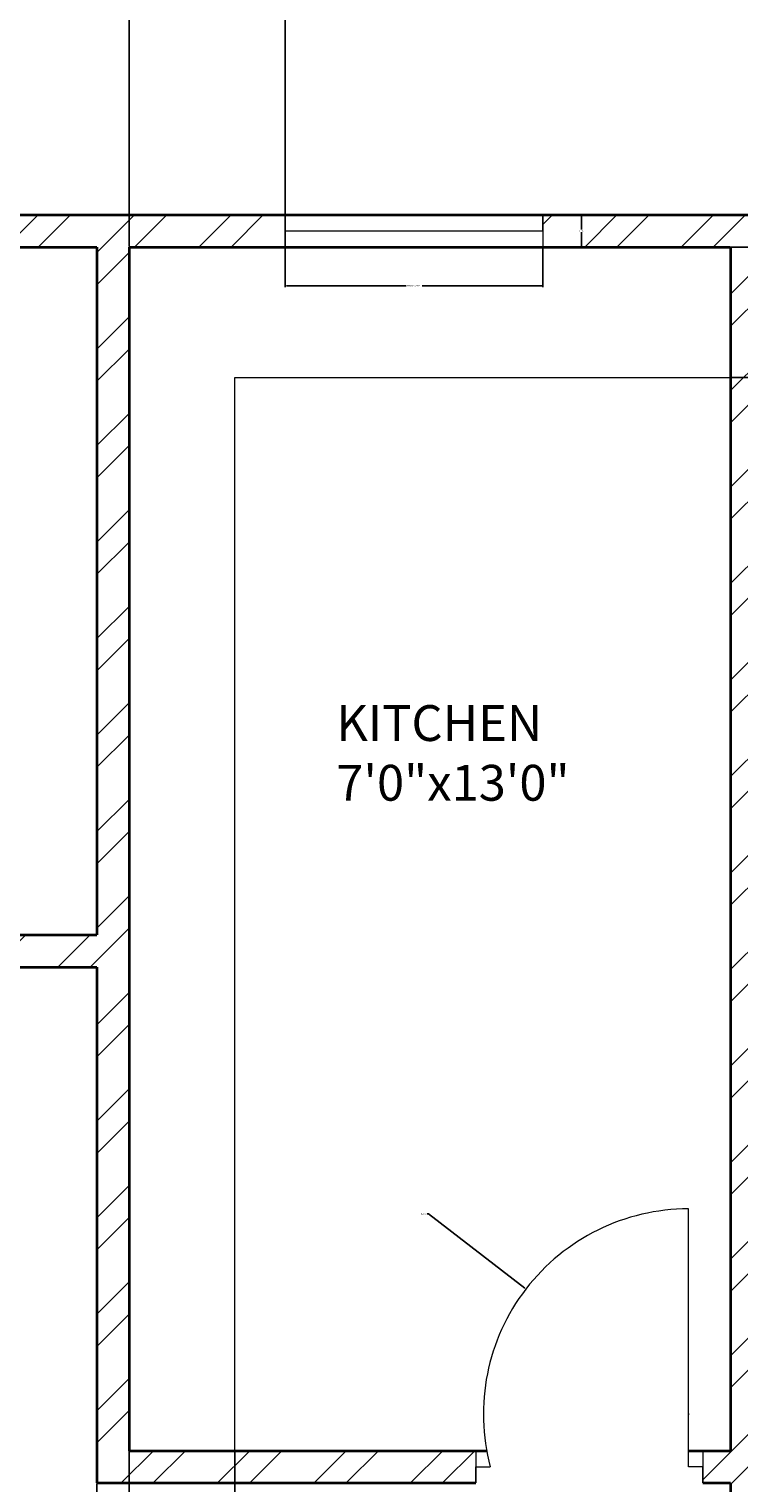
# Model space of a CAD drawing. Units: inches. Extents: x 392 to 1254, y 1207 to 2665.
# Tile 10 of 15: x 733 to 832, y 2052 to 2255. Entities that reach past the tile are written whole.
import ezdxf

# ---------------------------------------------------------------- set-up
doc = ezdxf.new("R2010")
doc.units = ezdxf.units.IN
for name, color, linetype, lineweight in [('A-ANNO-DIMS', 2, 'Continuous', 18), ('A-AREA-IDEN', 7, 'Continuous', 18), ('A-DOOR', 3, 'Continuous', 18), ('A-FLOR-FIXT', 9, 'Continuous', 18), ('A-GLAZ', 4, 'Continuous', 18), ('A-WALL', 7, 'Continuous', 35), ('A-WALL-PATT', 252, 'Continuous', 13)]:
    doc.layers.add(name, color=color, linetype=linetype, lineweight=lineweight)
doc.styles.get("Standard").update_dxf_attribs({"font": 'arial.ttf'})
doc.dimstyles.get("Standard").update_dxf_attribs({"dimtxt": 0.18, "dimasz": 0.18, "dimexe": 0.18, "dimexo": 0.0625, "dimgap": 0.09, "dimtad": 0, "dimtih": 1, "dimtoh": 1, "dimdec": 4, "dimzin": 0, "dimdsep": 46, "dimtxsty": 'Standard', "dimcen": 0.09, "dimadec": 0, "dimazin": 0, "dimtfac": 1, "dimtdec": 4, "dimtofl": 0, "dimtmove": 0, "dimatfit": 3, "dimfxl": 1, "dimtolj": 1, "dimtzin": 0, "dimarcsym": 0})

# ---------------------------------------------------------------- blocks, each defined once
blk = doc.blocks.new('WIN-36')
for p, q in [((0, 0), (0, 4.5)), ((0, 4.5), (0, 2.25)), ((36, 2.25), (36, 4.5)), ((36, 4.5), (36, 0)), ((0, 2.25), (36, 2.25))]:
    blk.add_line(p, q)
blk = doc.blocks.new('*D23')
at = {"layer": 'A-ANNO-DIMS', "color": 0, "lineweight": -2, "transparency": 16777216}
for p, q in [((768.58, 2224.73), (768.58, 2219.22)), ((804.58, 2224.73), (804.58, 2219.22)), ((768.76, 2219.4), (785.46, 2219.4)), ((804.4, 2219.4), (787.7, 2219.4))]:
    blk.add_line(p, q, dxfattribs=at)
at = {"layer": 'A-ANNO-DIMS', "color": 0, "transparency": 16777216}
for points in [[(768.76, 2219.43), (768.76, 2219.37), (768.58, 2219.4)], [(804.4, 2219.43), (804.4, 2219.37), (804.58, 2219.4)]]:
    blk.add_solid(points, dxfattribs=at)
at = {"layer": 'Defpoints', "color": 0, "transparency": 16777216}
for p in [(768.58, 2224.8), (804.58, 2224.8), (804.58, 2219.4)]:
    blk.add_point(p, dxfattribs=at)
at = {"layer": 'A-ANNO-DIMS', "color": 0, "transparency": 16777216, "insert": (786.58, 2219.4), "char_height": 0.18, "attachment_point": 5}
blk.add_mtext('\\A1;WINDOW 36 TYP.', dxfattribs=at)
blk = doc.blocks.new('*D24')
at = {"layer": 'A-ANNO-DIMS', "color": 0, "lineweight": -2, "transparency": 16777216}
for p, q in [((804.64, 2229.3), (810.16, 2229.3)), ((809.98, 2229.12), (809.98, 2227.23)), ((809.98, 2224.98), (809.98, 2226.86)), ((804.64, 2224.8), (810.16, 2224.8))]:
    blk.add_line(p, q, dxfattribs=at)
at = {"layer": 'A-ANNO-DIMS', "color": 0, "transparency": 16777216}
for points in [[(809.95, 2229.12), (810.01, 2229.12), (809.98, 2229.3)], [(809.95, 2224.98), (810.01, 2224.98), (809.98, 2224.8)]]:
    blk.add_solid(points, dxfattribs=at)
at = {"layer": 'Defpoints', "color": 0, "transparency": 16777216}
for p in [(804.58, 2229.3), (809.98, 2229.3), (804.58, 2224.8)]:
    blk.add_point(p, dxfattribs=at)
at = {"layer": 'A-ANNO-DIMS', "color": 0, "transparency": 16777216, "insert": (809.98, 2227.05), "char_height": 0.18, "attachment_point": 5}
blk.add_mtext('\\A1;5 TYP.', dxfattribs=at)
blk = doc.blocks.new('*D26')
at = {"layer": 'A-ANNO-DIMS', "color": 0, "lineweight": -2, "transparency": 16777216}
for p, q in [((541.22, 2229.3), (495, 2229.3)), ((495.18, 2229.12), (495.18, 1819.98)), ((495.18, 1410.48), (495.18, 1819.61)), ((753.23, 1410.3), (495, 1410.3))]:
    blk.add_line(p, q, dxfattribs=at)
at = {"layer": 'A-ANNO-DIMS', "color": 0, "transparency": 16777216}
for points in [[(495.15, 2229.12), (495.21, 2229.12), (495.18, 2229.3)], [(495.15, 1410.48), (495.21, 1410.48), (495.18, 1410.3)]]:
    blk.add_solid(points, dxfattribs=at)
at = {"layer": 'Defpoints', "color": 0, "transparency": 16777216}
for p in [(495.18, 2229.3), (541.28, 2229.3), (753.29, 1410.3)]:
    blk.add_point(p, dxfattribs=at)
at = {"layer": 'A-ANNO-DIMS', "color": 0, "transparency": 16777216, "insert": (495.18, 1819.8), "char_height": 0.18, "attachment_point": 5}
blk.add_mtext('\\A1;819', dxfattribs=at)
blk = doc.blocks.new('*D75')
at = {"layer": 'A-ANNO-DIMS', "color": 0, "lineweight": -2, "transparency": 16777216}
for p, q in [((746.78, 2056.73), (746.78, 1364.02)), ((742.28, 2052.23), (742.28, 1364.02)), ((742.46, 1364.2), (744.27, 1364.2)), ((746.6, 1364.2), (744.79, 1364.2))]:
    blk.add_line(p, q, dxfattribs=at)
at = {"layer": 'A-ANNO-DIMS', "color": 0, "transparency": 16777216}
for points in [[(742.46, 1364.23), (742.46, 1364.17), (742.28, 1364.2)], [(746.6, 1364.23), (746.6, 1364.17), (746.78, 1364.2)]]:
    blk.add_solid(points, dxfattribs=at)
at = {"layer": 'Defpoints', "color": 0, "transparency": 16777216}
for p in [(746.78, 2056.8), (742.28, 2052.3), (746.78, 1364.2)]:
    blk.add_point(p, dxfattribs=at)
at = {"layer": 'A-ANNO-DIMS', "color": 0, "transparency": 16777216, "insert": (744.53, 1364.2), "char_height": 0.18, "attachment_point": 5}
blk.add_mtext('\\A1;4.5', dxfattribs=at)
blk = doc.blocks.new('*D77')
at = {"layer": 'A-ANNO-DIMS', "color": 0, "lineweight": -2, "transparency": 16777216}
for p, q in [((746.78, 2224.86), (746.78, 2297.33)), ((768.58, 2224.86), (768.58, 2297.33)), ((746.96, 2297.15), (757.21, 2297.15)), ((768.4, 2297.15), (758.14, 2297.15))]:
    blk.add_line(p, q, dxfattribs=at)
at = {"layer": 'A-ANNO-DIMS', "color": 0, "transparency": 16777216}
for points in [[(746.96, 2297.18), (746.96, 2297.12), (746.78, 2297.15)], [(768.4, 2297.18), (768.4, 2297.12), (768.58, 2297.15)]]:
    blk.add_solid(points, dxfattribs=at)
at = {"layer": 'Defpoints', "color": 0, "transparency": 16777216}
for p in [(768.58, 2297.15), (746.78, 2224.8), (768.58, 2224.8)]:
    blk.add_point(p, dxfattribs=at)
at = {"layer": 'A-ANNO-DIMS', "color": 0, "transparency": 16777216, "insert": (757.68, 2297.15), "char_height": 0.18, "attachment_point": 5}
blk.add_mtext('\\A1;21.796', dxfattribs=at)
blk = doc.blocks.new('*D78')
at = {"layer": 'A-ANNO-DIMS', "color": 0, "lineweight": -2, "transparency": 16777216}
for p, q in [((746.78, 2056.73), (746.78, 1364.02)), ((761.56, 2056.73), (761.56, 1364.02)), ((746.96, 1364.2), (753.72, 1364.2)), ((761.38, 1364.2), (754.63, 1364.2))]:
    blk.add_line(p, q, dxfattribs=at)
at = {"layer": 'A-ANNO-DIMS', "color": 0, "transparency": 16777216}
for points in [[(746.96, 1364.23), (746.96, 1364.17), (746.78, 1364.2)], [(761.38, 1364.23), (761.38, 1364.17), (761.56, 1364.2)]]:
    blk.add_solid(points, dxfattribs=at)
at = {"layer": 'Defpoints', "color": 0, "transparency": 16777216}
for p in [(746.78, 2056.8), (761.56, 2056.8), (761.56, 1364.2)]:
    blk.add_point(p, dxfattribs=at)
at = {"layer": 'A-ANNO-DIMS', "color": 0, "transparency": 16777216, "insert": (754.17, 1364.2), "char_height": 0.18, "attachment_point": 5}
blk.add_mtext('\\A1;14.782', dxfattribs=at)
blk = doc.blocks.new('*D79')
at = {"layer": 'A-ANNO-DIMS', "color": 0, "lineweight": -2, "transparency": 16777216}
for p, q in [((830.84, 2224.8), (1171.06, 2224.8)), ((1170.88, 2224.62), (1170.88, 2215.87)), ((1170.88, 2206.76), (1170.88, 2215.5)), ((830.84, 2206.58), (1171.06, 2206.58))]:
    blk.add_line(p, q, dxfattribs=at)
at = {"layer": 'A-ANNO-DIMS', "color": 0, "transparency": 16777216}
for points in [[(1170.85, 2224.62), (1170.91, 2224.62), (1170.88, 2224.8)], [(1170.85, 2206.76), (1170.91, 2206.76), (1170.88, 2206.58)]]:
    blk.add_solid(points, dxfattribs=at)
at = {"layer": 'Defpoints', "color": 0, "transparency": 16777216}
for p in [(830.78, 2224.8), (1170.88, 2224.8), (830.78, 2206.58)]:
    blk.add_point(p, dxfattribs=at)
at = {"layer": 'A-ANNO-DIMS', "color": 0, "transparency": 16777216, "insert": (1170.88, 2215.69), "char_height": 0.18, "attachment_point": 5}
blk.add_mtext('\\A1;18.22', dxfattribs=at)
blk = doc.blocks.new('*D88')
at = {"layer": 'A-ANNO-DIMS', "color": 0, "lineweight": -2, "transparency": 16777216}
for p, q in [((788.39, 2089.85), (788.57, 2089.85)), ((788.57, 2089.85), (802.05, 2079.47)), ((824.82, 2061.89), (825, 2061.89)), ((824.91, 2061.8), (824.91, 2061.98))]:
    blk.add_line(p, q, dxfattribs=at)
at = {"layer": 'A-ANNO-DIMS', "color": 0, "transparency": 16777216}
blk.add_solid([(802.07, 2079.5), (802.04, 2079.45), (802.2, 2079.36)], dxfattribs=at)
at = {"layer": 'Defpoints', "color": 0, "transparency": 16777216}
for p in [(802.2, 2079.36), (824.91, 2061.89)]:
    blk.add_point(p, dxfattribs=at)
at = {"layer": 'A-ANNO-DIMS', "color": 0, "transparency": 16777216, "insert": (787.91, 2089.85), "char_height": 0.18, "attachment_point": 5}
blk.add_mtext('\\A1;R28.65', dxfattribs=at)

msp = doc.modelspace()

# ---------------------------------------------------------------- hatches: boundary and pattern name
at = {"layer": 'A-WALL-PATT'}
h = msp.add_hatch(dxfattribs=at)
h.set_pattern_fill('ANSI32', color=256)
h.paths.add_polyline_path([(579.5309, 2227.0453), (579.5309, 2229.2953), (541.2807, 2229.2953), (541.2807, 2182.3091), (545.7807, 2182.3091), (545.7807, 2224.7953), (579.5309, 2224.7953)])
h.paths.add_polyline_path([(655.4442, 2229.2953), (627.5309, 2229.2953), (627.5309, 2224.7953), (655.4442, 2224.7953), (655.4442, 2227.0453)])
h.paths.add_polyline_path([(703.0758, 2229.2953), (678.5257, 2229.2953), (678.5257, 2227.0453), (678.5257, 2224.7953), (689.7807, 2224.7953), (689.7807, 2158.6973), (694.2807, 2158.6973), (694.2807, 2224.7953), (703.0758, 2224.7953)])
h.paths.add_polyline_path([(768.5767, 2229.2953), (727.0758, 2229.2953), (727.0758, 2224.7953), (742.2807, 2224.7953), (742.2807, 2128.7953), (694.2807, 2128.7953), (694.2807, 2134.0554), (689.7807, 2134.0554), (689.7807, 2090.2854), (694.2807, 2090.2854), (694.2807, 2124.2953), (742.2807, 2124.2953), (742.2807, 2052.2953), (795.2124, 2052.2953), (795.2124, 2054.5453), (795.2124, 2056.7953), (746.7807, 2056.7953), (746.7807, 2224.7953), (768.5767, 2224.7953)])
h.paths.add_polyline_path([(867.5089, 2229.2953), (804.5767, 2229.2953), (804.5767, 2224.7953), (830.7807, 2224.7953), (830.7807, 2056.7953), (826.9066, 2056.7953), (826.9066, 2052.2953), (830.7807, 2052.2953), (830.7807, 1886.6777, -0.01766664), (830.8602, 1884.2953), (835.0818, 1884.2953, -0.04411348), (835.2807, 1889.9369), (835.2807, 2052.2953), (839.418, 2052.2953), (839.418, 2056.7953), (835.2807, 2056.7953), (835.2807, 2224.7953), (867.5089, 2224.7953)])
h.paths.add_polyline_path([(939.8604, 2229.2953), (903.5089, 2229.2953), (903.5089, 2227.0453), (903.5089, 2224.7953), (919.2807, 2224.7953), (919.2807, 2056.7953), (870.6499, 2056.7953), (870.6499, 2052.2953), (923.7807, 2052.2953), (923.7807, 2124.2953), (971.7807, 2124.2953), (971.7807, 2089.7112), (974.0307, 2089.7112), (976.2807, 2089.7112), (976.2807, 2133.56), (974.0307, 2133.56), (971.7807, 2133.56), (971.7807, 2128.7953), (923.7807, 2128.7953), (923.7807, 2224.7953), (939.8604, 2224.7953)])
h.paths.add_polyline_path([(1124.7807, 2229.2953), (1009.403, 2229.2953), (1009.403, 2224.7953), (1120.2807, 2224.7953), (1120.2807, 2184.7605), (1124.7807, 2184.7605)])
h.paths.add_polyline_path([(1124.7807, 2124.7605), (1120.2807, 2124.7605), (1120.2807, 2056.7953), (976.2807, 2056.7953), (976.2807, 2061.471), (971.7807, 2061.471), (971.7807, 2047.7483), (974.0307, 2047.7483), (976.2807, 2047.7483), (976.2807, 2052.2953), (1120.2807, 2052.2953), (1120.2807, 1992.457), (1124.7807, 1992.457)])
h.paths.add_polyline_path([(1124.7807, 1932.457), (1122.5307, 1932.457), (1120.2807, 1932.457), (1120.2807, 1884.2953), (976.2807, 1884.2953), (976.2807, 2019.9536), (971.7807, 2019.9536), (971.7807, 1884.2953), (869.0911, 1884.2953), (869.0911, 1879.7953), (971.7807, 1879.7953), (1013.7807, 1879.7953), (1013.7807, 1831.7953), (971.7807, 1831.7953), (971.7807, 1822.3831), (974.0307, 1822.3831), (976.2807, 1822.3831), (976.2807, 1827.2953), (1013.7807, 1827.2953), (1025.6191, 1827.2953), (1025.6191, 1829.5453), (1025.6191, 1831.7953), (1018.2807, 1831.7953), (1018.2807, 1879.7953), (1120.2807, 1879.7953), (1120.2807, 1866.9192), (1124.7807, 1866.9192)])
h.paths.add_polyline_path([(1124.7807, 1842.9192), (1122.5307, 1842.9192), (1120.2807, 1842.9192), (1120.2807, 1831.7953), (1050.2021, 1831.7953), (1050.2021, 1827.2953), (1120.2807, 1827.2953), (1120.2807, 1781.4559), (1124.7807, 1781.4559)])
h.paths.add_polyline_path([(976.2807, 1790.8718), (971.7807, 1790.8718), (971.7807, 1648.3339), (976.2807, 1648.3339), (976.2807, 1654.7953), (1120.2807, 1654.7953), (1120.2807, 1626.3807), (1124.7807, 1626.3807), (1124.7807, 1721.4559), (1120.2807, 1721.4559), (1120.2807, 1659.2953), (976.2807, 1659.2953)])
h.paths.add_polyline_path([(1124.7807, 1566.3807), (1120.2807, 1566.3807), (1120.2807, 1486.7953), (1101.07, 1486.7953), (1101.07, 1482.2953), (1124.7807, 1482.2953)])
h.paths.add_polyline_path([(1041.07, 1484.5453), (1041.07, 1486.7953), (1006.2807, 1486.7953), (1006.2807, 1484.5453), (1006.2807, 1482.2953), (1041.07, 1482.2953)])
h.paths.add_polyline_path([(976.2807, 1617.5497), (974.0307, 1617.5497), (971.7807, 1617.5497), (971.7807, 1599.2953), (965.8041, 1599.2953), (965.8041, 1594.7953), (971.7807, 1594.7953), (971.7807, 1486.7953), (954.1249, 1486.7953), (954.1249, 1482.2953), (981.5717, 1482.2953), (981.5717, 1484.5453), (981.5717, 1486.7953), (976.2807, 1486.7953)])
h.paths.add_polyline_path([(930.1249, 1486.7953), (887.7807, 1486.7953), (887.7807, 1594.7953), (941.9141, 1594.7953), (941.9141, 1597.0453), (941.9141, 1599.2953), (887.7807, 1599.2953), (887.7807, 1659.2953), (863.5916, 1659.2953), (863.5916, 1654.7953), (883.2807, 1654.7953), (883.2807, 1438.7953), (782.7807, 1438.7953), (782.7807, 1486.7953), (782.7807, 1654.7953), (800.1309, 1654.7953), (800.1309, 1657.0453), (800.1309, 1659.2953), (778.2807, 1659.2953), (778.2807, 1599.2953), (721.7333, 1599.2953), (721.7333, 1597.0453), (721.7333, 1594.7953), (778.2807, 1594.7953), (778.2807, 1486.7953), (729.598, 1486.7953), (729.598, 1482.2953), (753.2885, 1482.2953), (753.2885, 1410.2953), (922.9852, 1410.2953), (922.9852, 1482.2953), (930.1249, 1482.2953)])
h.paths.add_polyline_path([(918.4852, 1482.2953), (918.4852, 1414.7953), (757.7885, 1414.7953), (757.7885, 1482.2953), (778.2807, 1482.2953), (778.2807, 1434.2953), (782.7807, 1434.2953), (887.7807, 1434.2953), (887.7807, 1438.7953), (887.7807, 1482.2953)], flags=16)
h.paths.add_polyline_path([(694.2807, 1594.7953), (700.4169, 1594.7953), (700.4169, 1597.0453), (700.4169, 1599.2953), (694.2807, 1599.2953), (694.2807, 1617.7503), (692.0307, 1617.7503), (689.7807, 1617.7503), (689.7807, 1486.7953), (682.7672, 1486.7953), (682.7672, 1482.2953), (705.598, 1482.2953), (705.598, 1484.5453), (705.598, 1486.7953), (694.2807, 1486.7953)])
h.paths.add_polyline_path([(545.7807, 1654.7953), (689.7807, 1654.7953), (689.7807, 1649.7691), (694.2807, 1649.7691), (694.2807, 1789.3981), (692.0307, 1789.3981), (689.7807, 1789.3981), (689.7807, 1659.2953), (545.7807, 1659.2953), (545.7807, 1714.4681), (543.5307, 1714.4681), (541.2807, 1714.4681), (541.2807, 1482.2953), (567.0628, 1482.2953), (567.0628, 1484.5453), (567.0628, 1486.7953), (545.7807, 1486.7953)])
h.paths.add_polyline_path([(545.7807, 1827.2953), (620.2247, 1827.2953), (620.2247, 1829.5453), (620.2247, 1831.7953), (545.7807, 1831.7953), (545.7807, 1846.8518), (541.2807, 1846.8518), (541.2807, 1774.4681), (545.7807, 1774.4681)])
h.paths.add_polyline_path([(797.0944, 1884.2953), (694.2807, 1884.2953), (694.2807, 2019.0288), (692.0307, 2019.0288), (689.7807, 2019.0288), (689.7807, 1884.2953), (545.7807, 1884.2953), (545.7807, 1951.8244), (541.2807, 1951.8244), (541.2807, 1870.8518), (543.5307, 1870.8518), (545.7807, 1870.8518), (545.7807, 1879.7953), (647.7807, 1879.7953), (647.7807, 1831.7953), (642.6413, 1831.7953), (642.6413, 1827.2953), (652.2807, 1827.2953), (689.7807, 1827.2953), (689.7807, 1821.0531), (694.2807, 1821.0531), (694.2807, 1831.7953), (652.2807, 1831.7953), (652.2807, 1879.7953), (797.0944, 1879.7953), (797.0944, 1882.0453)])
h.paths.add_polyline_path([(545.7807, 2122.3091), (541.2807, 2122.3091), (541.2807, 2011.8244), (543.5307, 2011.8244), (545.7807, 2011.8244), (545.7807, 2052.2953), (689.7807, 2052.2953), (689.7807, 2048.2048), (694.2807, 2048.2048), (694.2807, 2061.3129), (692.0307, 2061.3129), (689.7807, 2061.3129), (689.7807, 2056.7953), (545.7807, 2056.7953)])

# ---------------------------------------------------------------- linework, layer by layer
at = {"layer": 'A-DOOR'}
for p, q in [((824.9066, 2054.5453), (824.9066, 2090.5453)), ((795.2124, 2056.7953), (795.2124, 2052.2953)), ((826.9066, 2056.7953), (826.9066, 2052.2953)), ((795.2124, 2052.2953), (795.2124, 2054.5453)), ((795.2124, 2054.5453), (797.2124, 2054.5453)), ((826.9066, 2054.5453), (824.9066, 2054.5453)), ((826.9066, 2052.2953), (826.9066, 2054.5453))]:
    msp.add_line(p, q, dxfattribs=at)
msp.add_arc((824.9066, 2061.8929), 28.6524, 90, 194.858861, dxfattribs=at)
at = {"layer": 'A-FLOR-FIXT'}
for p, q in [((761.5625, 2056.7953), (761.5625, 2206.5771)), ((761.5625, 2206.5771), (830.7807, 2206.5771))]:
    msp.add_line(p, q, dxfattribs=at)
at = {"layer": 'A-WALL'}
for p, q in [((676.5257, 2229.2953), (985.8869, 2229.2953)), ((694.2807, 2224.7953), (742.2807, 2224.7953)), ((742.2807, 2224.7953), (742.2807, 2128.7953)), ((746.7807, 2224.7953), (746.7807, 2056.7953)), ((746.7807, 2224.7953), (830.7807, 2224.7953)), ((830.7807, 2224.7953), (830.7807, 2056.7953)), ((694.2807, 2128.7953), (742.2807, 2128.7953)), ((694.2807, 2124.2953), (742.2807, 2124.2953)), ((742.2807, 2124.2953), (742.2807, 2052.2953)), ((746.7807, 2056.7953), (796.7113, 2056.7953)), ((824.9066, 2056.7953), (830.7807, 2056.7953)), ((742.2807, 2052.2953), (795.2124, 2052.2953)), ((826.9066, 2052.2953), (830.7807, 2052.2953)), ((830.7807, 2052.2953), (830.7807, 1884.2953))]:
    msp.add_line(p, q, dxfattribs=at)

# ---------------------------------------------------------------- block references
at = {"layer": 'A-GLAZ'}
msp.add_blockref('WIN-36', (768.577, 2224.795), dxfattribs=at)

# ---------------------------------------------------------------- texts
at = {"layer": 'A-AREA-IDEN', "insert": (775.7174, 2160.8598), "char_height": 5, "attachment_point": 1}
msp.add_mtext_dynamic_manual_height_columns('KITCHEN\\P7\'0"x13\'0"', width=129.506855, gutter_width=12.5, heights=[0], dxfattribs=at)

# ---------------------------------------------------------------- dimensions: what is measured, and where the dimension line sits
at = {"layer": 'A-ANNO-DIMS'}
for base, p1, p2, override, picture, middle in [((768.5767, 2297.1453), (746.7807, 2224.7953), (768.5767, 2224.7953), {"dimdec": 3, "dimlfac": 1, "dimrnd": 0, "dimzin": 0, "dimdsep": 46, "dimlunit": 2}, '*D77', (757.6787, 2297.1453)), ((746.7807, 1364.1953), (742.2807, 2052.2953), (746.7807, 2056.7953), {"dimdec": 1, "dimlfac": 1, "dimrnd": 0, "dimzin": 0, "dimdsep": 46, "dimlunit": 2}, '*D75', (744.5307, 1364.1953)), ((761.5625, 1364.1953), (746.7807, 2056.7953), (761.5625, 2056.7953), {"dimdec": 3, "dimlfac": 1, "dimrnd": 0, "dimzin": 0, "dimdsep": 46, "dimlunit": 2}, '*D78', (754.1716, 1364.1953))]:
    dim = msp.add_linear_dim(base=base, p1=p1, p2=p2, dimstyle='Standard', override=override, dxfattribs=at)
    dim.commit()
    dim.dimension.update_dxf_attribs({"geometry": picture, "text_midpoint": middle})
for base, p1, p2, override, picture, middle in [((495.1807, 2229.2953), (753.2885, 1410.2953), (541.2807, 2229.2953), {"dimdec": 0, "dimlfac": 1, "dimrnd": 0, "dimzin": 0, "dimdsep": 46, "dimlunit": 2}, '*D26', (495.1807, 1819.7953)), ((1170.8807, 2224.7953), (830.7807, 2206.5771), (830.7807, 2224.7953), {"dimdec": 2, "dimlfac": 1, "dimrnd": 0, "dimzin": 0, "dimdsep": 46, "dimlunit": 2}, '*D79', (1170.8807, 2215.6862))]:
    dim = msp.add_linear_dim(base=base, p1=p1, p2=p2, angle=90, dimstyle='Standard', override=override, dxfattribs=at)
    dim.commit()
    dim.dimension.update_dxf_attribs({"geometry": picture, "text_midpoint": middle})
dim = msp.add_linear_dim(base=(809.9766691174, 2229.2953173571), p1=(804.5766691174, 2224.7953173571), p2=(804.5766691174, 2229.2953173571), angle=90, text='<> TYP.', dimstyle='Standard', override={"dimdec": 0, "dimlfac": 1, "dimrnd": 0, "dimzin": 0, "dimdsep": 46, "dimlunit": 2}, dxfattribs=at)
dim.commit()
dim.dimension.update_dxf_attribs({"geometry": '*D24', "text_midpoint": (809.9766691174, 2227.0453173571)})
dim = msp.add_linear_dim(base=(804.5767, 2219.3953), p1=(768.5767, 2224.7953), p2=(804.5767, 2224.7953), text='WINDOW <> TYP.', dimstyle='Standard', override={"dimdec": 0, "dimlfac": 1, "dimrnd": 0, "dimzin": 0, "dimdsep": 46, "dimlunit": 2}, dxfattribs=at)
dim.commit()
dim.dimension.update_dxf_attribs({"geometry": '*D23', "text_midpoint": (786.5767, 2219.3953)})
dim = msp.add_radius_dim(center=(824.9066, 2061.8929), mpoint=(802.1966, 2079.3633), dimstyle='Standard', override={"dimdec": 2, "dimlfac": 1, "dimrnd": 0, "dimzin": 0, "dimdsep": 46, "dimlunit": 2}, dxfattribs=at)
dim.commit()
dim.dimension.update_dxf_attribs({"geometry": '*D88', "text_midpoint": (787.9101, 2089.8455), "dimtype": 164})

doc.saveas('drawing.dxf')
